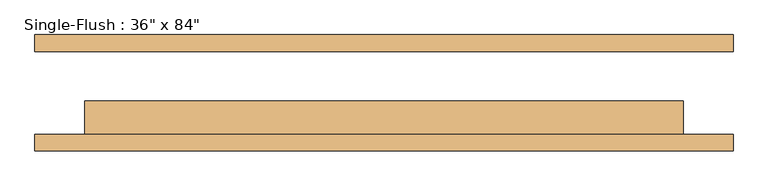
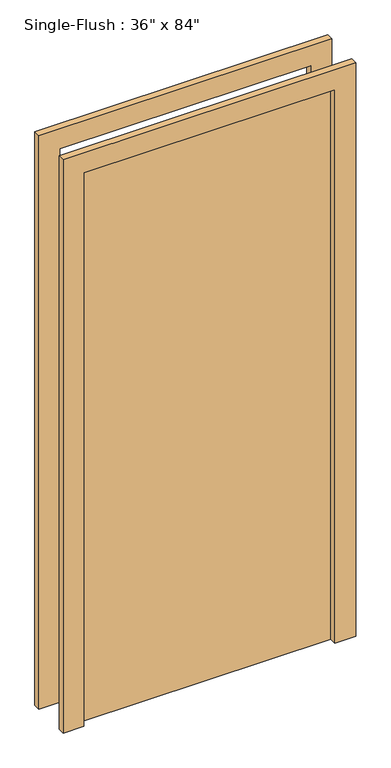
"""IFC4 building model written with IfcOpenShell, lengths in millimetres: door geometry."""

from ifc_helpers import new_model, si_unit, frame, origin, origin_with_axes, place, context, project, spatial, polyline, outline, extrude, source, transform, mapped, element, save


def door_a3eb833a(model_context):
    return source(origin(), model_context, "Body", "SweptSolid", [
        extrude(outline(polyline([(2209.8, -533.4), (0.0, -533.4), (0.0, -457.2), (2133.6, -457.2), (2133.6, 457.2), (0.0, 457.2), (0.0, 533.4), (2209.8, 533.4), (2209.8, -533.4)])), frame((0.0, -88.9, 0.0), z_axis=(0.0, 1.0, 0.0), x_axis=(0.0, 0.0, 1.0)), (0.0, 0.0, 1.0), 25.4),
        extrude(outline(polyline([(2209.8, 533.4), (2209.8, -533.4), (0.0, -533.4), (0.0, -457.2), (2133.6, -457.2), (2133.6, 457.2), (0.0, 457.2), (0.0, 533.4), (2209.8, 533.4)])), frame((0.0, 63.5, 0.0), z_axis=(0.0, 1.0, 0.0), x_axis=(0.0, 0.0, 1.0)), (0.0, 0.0, 1.0), 25.4),
        extrude(outline(polyline([(457.2, -12.7), (457.2, -63.5), (-457.2, -63.5), (-457.2, -12.7), (457.2, -12.7)])), origin_with_axes(), (0.0, 0.0, 1.0), 2133.6),
    ])


if __name__ == "__main__":
    model = new_model("IFC4")
    model_context = context("Model", 3, world=origin())
    ifc_project = project(units=[si_unit("LENGTHUNIT", "METRE", prefix="MILLI")], contexts=[model_context])
    site = spatial("IfcSite", under=ifc_project)
    building = spatial("IfcBuilding", under=site)
    placement = place(None, origin())
    door_shape = door_a3eb833a(model_context)
    element("IfcDoor", 1, ObjectType="Single-Flush : 36\" x 84\"", at=placement, inside=building, context=model_context, shape_type="MappedRepresentation", body=[
        mapped(door_shape, transform((0.0, 0.0, 0.0), x_axis=(1.0, 0.0, 0.0), y_axis=(0.0, 1.0, 0.0), z_axis=(0.0, 0.0, 1.0))),
    ])
    save(model, "model.ifc")

# Revit data of these elements
# Type "Single-Flush : 36\" x 84\""
#   Type Mark = "1"
#   Construction Type Id = "MDOOR"
#   Assembly Code = "C1020"
#   Analytic Construction = "Metal"
#   Thickness = 0' - 2"
#   Heat Transfer Coefficient (U) = 0.651978 BTU/(h·ft²·°F)
#   Height = 7' - 0"
#   Trim Projection Ext = 0' - 1"
#   Trim Projection Int = 0' - 1"
#   Trim Width = 0' - 3"
#   Width = 3' - 0"
#   Define Thermal Properties by = 1
#   Define Thermal Properties by = 1
#   Door Material = Door - Panel
#   Frame Material = Door - Frame
#   Visual Light Transmittance = 0
#   Solar Heat Gain Coefficient = 0
#   Function = (empty or 0)
#   Wall Closure = (empty or 0)
# Element 1 (IfcDoor, "Single-Flush : 36\" x 84\"")
#   Materials on its faces: "Door - Frame", "Door - Panel"
# Materials
#   "Door - Panel": class "Wood", colour RGB 210 159 95, transparency 0, Cost = 0
#   "Door - Frame": colour RGB 118 70 51, transparency 0, Cost = 0
